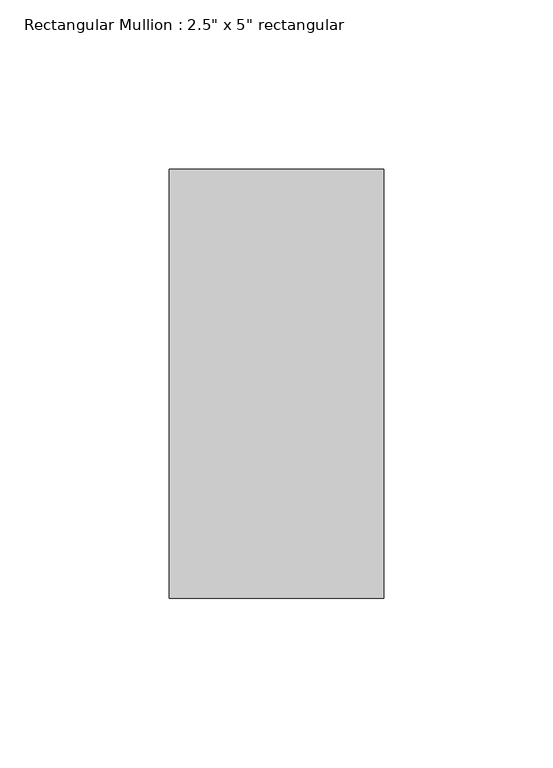
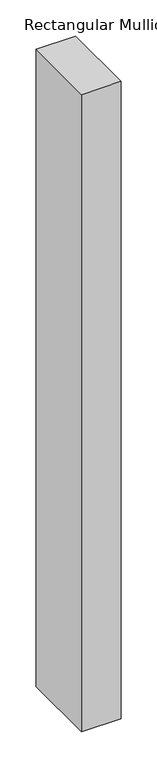
"""IFC4 building model written with IfcOpenShell, lengths in millimetres: member geometry."""

from ifc_helpers import new_model, si_unit, frame, origin, place, context, project, spatial, polyline, outline, extrude, source, transform, mapped, element, save


def member_ade69111(model_context):
    return source(origin(), model_context, "Body", "SweptSolid", [
        extrude(outline(polyline([(31.75, 63.5), (31.75, -63.5), (-31.75, -63.5), (-31.75, 63.5), (31.75, 63.5)])), frame((0.0, 0.0, -1079.7501856), z_axis=(0.0, 0.0, 1.0), x_axis=(1.0, 0.0, 0.0)), (0.0, 0.0, 1.0), 1079.7501856),
    ])


if __name__ == "__main__":
    model = new_model("IFC4")
    model_context = context("Model", 3, world=origin())
    ifc_project = project(units=[si_unit("LENGTHUNIT", "METRE", prefix="MILLI")], contexts=[model_context])
    site = spatial("IfcSite", under=ifc_project)
    building = spatial("IfcBuilding", under=site)
    placement = place(None, origin())
    member_shape = member_ade69111(model_context)
    element("IfcMember", 1, ObjectType="Rectangular Mullion : 2.5\" x 5\" rectangular", at=placement, inside=building, context=model_context, shape_type="MappedRepresentation", body=[
        mapped(member_shape, transform((0.0, 0.0, 0.0), x_axis=(1.0, 0.0, 0.0), y_axis=(0.0, 1.0, 0.0), z_axis=(0.0, 0.0, 1.0))),
    ])
    save(model, "model.ifc")

# Revit data of these elements
# Type "Rectangular Mullion : 2.5\" x 5\" rectangular"
#   built-in parameter 1007304 = 0.416667 (stored number, unit not read)
#   built-in parameter 1007301 = 0.104167 (stored number, unit not read)
#   built-in parameter 1007300 = 0.104167 (stored number, unit not read)
# Element 1 (IfcMember, "Rectangular Mullion : 2.5\" x 5\" rectangular")
#   Materials on its faces: "Aluminum"
# Materials
#   "Aluminum": class "Metal", colour RGB 247 247 247, transparency 0, Description = "Aluminum 6061", Cost = 0
